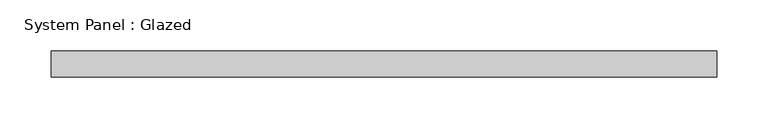
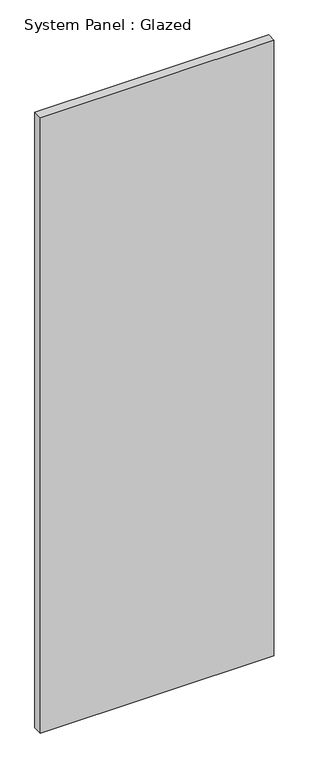
"""IFC4 building model written with IfcOpenShell, lengths in millimetres: plate geometry, System Panel : Glazed."""

from ifc_helpers import new_model, si_unit, origin, origin_with_axes, place, context, project, spatial, polyline, outline, extrude, source, transform, mapped, element, save


def system_panel_glazed_d2c96357(model_context):
    return source(origin(), model_context, "Body", "SweptSolid", [
        extrude(outline(polyline([(323.85, 19.05), (-323.85, 19.05), (-323.85, 44.45), (323.85, 44.45), (323.85, 19.05)])), origin_with_axes(), (0.0, 0.0, 1.0), 1804.193737),
    ])


if __name__ == "__main__":
    model = new_model("IFC4")
    model_context = context("Model", 3, world=origin())
    ifc_project = project(units=[si_unit("LENGTHUNIT", "METRE", prefix="MILLI")], contexts=[model_context])
    site = spatial("IfcSite", under=ifc_project)
    building = spatial("IfcBuilding", under=site)
    placement = place(None, origin())
    system_panel_glazed_shape = system_panel_glazed_d2c96357(model_context)
    element("IfcPlate", 1, ObjectType="System Panel : Glazed", at=placement, inside=building, context=model_context, shape_type="MappedRepresentation", body=[
        mapped(system_panel_glazed_shape, transform((0.0, 0.0, 0.0), x_axis=(1.0, 0.0, 0.0), y_axis=(0.0, 1.0, 0.0), z_axis=(0.0, 0.0, 1.0))),
    ])
    save(model, "model.ifc")

# Revit data of these elements
# Type "System Panel : Glazed"
#   Construction Type Id = "GSP4R"
#   Analytic Construction = "1/8 in Pilkington single glazing"
#   Visual Light Transmittance = 0.9
#   Solar Heat Gain Coefficient = 0.86
#   Heat Transfer Coefficient (U) = 1.18115 BTU/(h·ft²·°F)
#   Define Thermal Properties by = 1
# Element 1 (IfcPlate, "System Panel : Glazed")
#   Materials on its faces: "Glass"
# Materials
#   "Glass": class "Glass", colour RGB 0 128 192, transparency 0.75, Description = "Soda Lime Glass", Cost = 0
